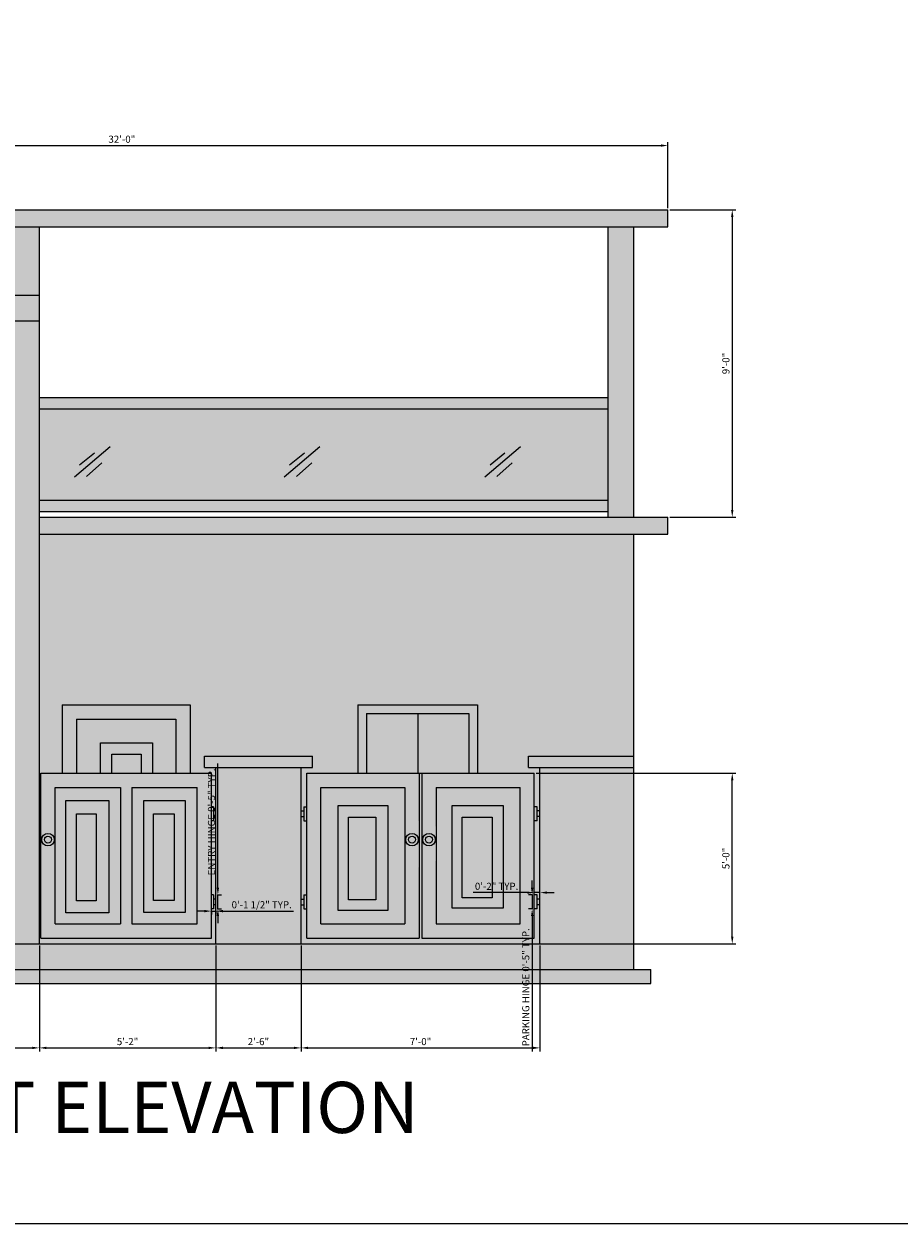
# Model space of a CAD drawing. Units: inches. Extents: x 2169 to 10664, y 1669 to 6352.
# Tile 2 of 17: x 2403 to 2710, y 1669 to 2091. Entities that reach past the tile are written whole.
import ezdxf

# ---------------------------------------------------------------- set-up
doc = ezdxf.new("R2010")
doc.units = ezdxf.units.IN
for name, color, linetype, lineweight in [('A-ANNO-DIMS', 3, 'Continuous', 18), ('A-ANNO-TITL', 3, 'Continuous', 25), ('A-ANNO-TTLB', 7, 'Continuous', 25), ('A-ELEV', 7, 'Continuous', 25), ('A-ELEV-CONC-PATT', 85, 'Continuous', 13), ('A-ELEV-GATE', 7, 'Continuous', 18), ('A-ELEV-GATE-PATT', 252, 'Continuous', 13), ('A-ELEV-OPEN', 7, 'Continuous', 18), ('A-ELEV-OPEN-PATT', 9, 'Continuous', 13), ('A-ELEV-PATT', 253, 'Continuous', 13)]:
    doc.layers.add(name, color=color, linetype=linetype, lineweight=lineweight)
doc.styles.get("Standard").update_dxf_attribs({"font": 'arial.ttf'})
doc.dimstyles.new('ISO-25', dxfattribs={"dimtxt": 2.5, "dimasz": 2.5, "dimexe": 1.25, "dimexo": 0.625, "dimtad": 1, "dimdec": 0, "dimlunit": 3, "dimtxsty": 'Standard', "dimcen": 2.5, "dimadec": 0, "dimazin": 0, "dimtfac": 1, "dimtdec": 0, "dimtmove": 0, "dimatfit": 3, "dimfxl": 1, "dimarcsym": 0})

# ---------------------------------------------------------------- blocks, each defined once
blk = doc.blocks.new('GLASS-MARK-A')
for p, q in [((0, 0), (12.55, 10.69)), ((1.85, 4.25), (7.07, 8.47)), ((4.25, 0.12), (9.7, 4.88))]:
    blk.add_line(p, q)
blk = doc.blocks.new('GATE-HINGE-1')
for p, q in [((0.75, 5), (0, 5)), ((0.75, 5), (0.75, 0)), ((0.75, 0), (0, 0)), ((1.5, 3.5), (0.75, 3.5)), ((1.5, 1.5), (0.75, 1.5))]:
    blk.add_line(p, q)
blk = doc.blocks.new('GATE-HINGE-2')
for p, q in [((1, 5), (2, 5)), ((1, 5), (1, 0)), ((0, 3.5), (1, 3.5)), ((0, 1.5), (1, 1.5)), ((1, 0), (2, 0))]:
    blk.add_line(p, q)
blk = doc.blocks.new('GATE-PULL-ROUND')
for radius in [2.2, 1.2]:
    blk.add_circle((2.21, 2.21), radius)
blk = doc.blocks.new('*D69')
at = {"layer": 'A-ANNO-DIMS', "color": 0, "lineweight": -2, "transparency": 16777216}
for p, q in [((2581.31, 1787.58), (2581.31, 1790.08)), ((2581.43, 1785.08), (2580.06, 1785.08)), ((2581.31, 1785.08), (2581.31, 1780.08)), ((2581.43, 1780.08), (2580.06, 1780.08)), ((2581.31, 1777.58), (2581.31, 1729.99))]:
    blk.add_line(p, q, dxfattribs=at)
at = {"layer": 'A-ANNO-DIMS', "color": 0, "transparency": 16777216}
for points in [[(2580.89, 1787.58), (2581.73, 1787.58), (2581.31, 1785.08)], [(2580.89, 1777.58), (2581.73, 1777.58), (2581.31, 1780.08)]]:
    blk.add_solid(points, dxfattribs=at)
at = {"layer": 'Defpoints', "color": 0, "transparency": 16777216}
for p in [(2582.06, 1785.08), (2581.31, 1780.08), (2582.06, 1780.08)]:
    blk.add_point(p, dxfattribs=at)
at = {"layer": 'A-ANNO-DIMS', "color": 0, "transparency": 16777216, "insert": (2579.39, 1752.54), "char_height": 2.5, "attachment_point": 5, "rotation": 90}
blk.add_mtext('PARKING HINGE 0\'-5" TYP.', dxfattribs=at)
blk = doc.blocks.new('*D70')
at = {"layer": 'A-ANNO-DIMS', "color": 0, "lineweight": -2, "transparency": 16777216}
for p, q in [((2579.56, 1785.83), (2560.57, 1785.83)), ((2582.06, 1785.7), (2582.06, 1787.08)), ((2584.06, 1785.83), (2582.06, 1785.83)), ((2584.06, 1785.7), (2584.06, 1787.08)), ((2586.56, 1785.83), (2589.06, 1785.83))]:
    blk.add_line(p, q, dxfattribs=at)
at = {"layer": 'A-ANNO-DIMS', "color": 0, "transparency": 16777216}
for points in [[(2579.56, 1786.24), (2579.56, 1785.41), (2582.06, 1785.83)], [(2586.56, 1786.24), (2586.56, 1785.41), (2584.06, 1785.83)]]:
    blk.add_solid(points, dxfattribs=at)
at = {"layer": 'Defpoints', "color": 0, "transparency": 16777216}
for p in [(2582.06, 1785.83), (2582.06, 1785.08), (2584.06, 1785.08)]:
    blk.add_point(p, dxfattribs=at)
at = {"layer": 'A-ANNO-DIMS', "color": 0, "transparency": 16777216, "insert": (2568.81, 1787.73), "char_height": 2.5, "attachment_point": 5}
blk.add_mtext('0\'-2" TYP.', dxfattribs=at)
blk = doc.blocks.new('*D79')
at = {"layer": 'A-ANNO-DIMS', "color": 0, "lineweight": -2, "transparency": 16777216}
for p, q in [((2470.81, 1787.58), (2470.81, 1831.27)), ((2470.68, 1785.08), (2472.06, 1785.08)), ((2470.81, 1780.08), (2470.81, 1785.08)), ((2470.68, 1780.08), (2472.06, 1780.08)), ((2470.81, 1777.58), (2470.81, 1775.08))]:
    blk.add_line(p, q, dxfattribs=at)
at = {"layer": 'A-ANNO-DIMS', "color": 0, "transparency": 16777216}
for points in [[(2470.39, 1787.58), (2471.23, 1787.58), (2470.81, 1785.08)], [(2470.39, 1777.58), (2471.23, 1777.58), (2470.81, 1780.08)]]:
    blk.add_solid(points, dxfattribs=at)
at = {"layer": 'Defpoints', "color": 0, "transparency": 16777216}
for p in [(2470.06, 1785.08), (2470.81, 1785.08), (2470.06, 1780.08)]:
    blk.add_point(p, dxfattribs=at)
at = {"layer": 'A-ANNO-DIMS', "color": 0, "transparency": 16777216, "insert": (2468.89, 1810.68), "char_height": 2.5, "attachment_point": 5, "rotation": 90}
blk.add_mtext('ENTRY HINGE 0\'-5" TYP.', dxfattribs=at)
blk = doc.blocks.new('*D80')
at = {"layer": 'A-ANNO-DIMS', "color": 0, "lineweight": -2, "transparency": 16777216}
for p, q in [((2466.06, 1779.33), (2463.56, 1779.33)), ((2468.56, 1779.45), (2468.56, 1778.08)), ((2468.56, 1779.33), (2470.06, 1779.33)), ((2470.06, 1779.45), (2470.06, 1778.08)), ((2472.56, 1779.33), (2497.37, 1779.33))]:
    blk.add_line(p, q, dxfattribs=at)
at = {"layer": 'A-ANNO-DIMS', "color": 0, "transparency": 16777216}
for points in [[(2466.06, 1779.74), (2466.06, 1778.91), (2468.56, 1779.33)], [(2472.56, 1779.74), (2472.56, 1778.91), (2470.06, 1779.33)]]:
    blk.add_solid(points, dxfattribs=at)
at = {"layer": 'Defpoints', "color": 0, "transparency": 16777216}
for p in [(2468.56, 1780.08), (2470.06, 1780.08), (2470.06, 1779.33)]:
    blk.add_point(p, dxfattribs=at)
at = {"layer": 'A-ANNO-DIMS', "color": 0, "transparency": 16777216, "insert": (2486.22, 1781.25), "char_height": 2.5, "attachment_point": 5}
blk.add_mtext('0\'-1 1/2" TYP.', dxfattribs=at)
blk = doc.blocks.new('*D93')
at = {"layer": 'A-ANNO-DIMS', "color": 0, "lineweight": -2, "transparency": 16777216}
for p, q in [((2245.06, 2026.47), (2245.06, 2049.69)), ((2247.56, 2048.44), (2626.56, 2048.44)), ((2629.06, 2026.47), (2629.06, 2049.69))]:
    blk.add_line(p, q, dxfattribs=at)
at = {"layer": 'A-ANNO-DIMS', "color": 0, "transparency": 16777216}
for points in [[(2247.56, 2048.86), (2247.56, 2048.03), (2245.06, 2048.44)], [(2626.56, 2048.86), (2626.56, 2048.03), (2629.06, 2048.44)]]:
    blk.add_solid(points, dxfattribs=at)
at = {"layer": 'Defpoints', "color": 0, "transparency": 16777216}
for p in [(2629.06, 2048.44), (2245.06, 2025.84), (2629.06, 2025.84)]:
    blk.add_point(p, dxfattribs=at)
at = {"layer": 'A-ANNO-DIMS', "color": 0, "transparency": 16777216, "insert": (2437.06, 2050.35), "char_height": 2.5, "attachment_point": 5}
blk.add_mtext('32\'-0"', dxfattribs=at)
blk = doc.blocks.new('*D94')
at = {"layer": 'A-ANNO-DIMS', "color": 0, "lineweight": -2, "transparency": 16777216}
for p, q in [((2629.68, 2025.84), (2652.91, 2025.84)), ((2651.66, 2023.34), (2651.66, 1920.34)), ((2629.68, 1917.84), (2652.91, 1917.84))]:
    blk.add_line(p, q, dxfattribs=at)
at = {"layer": 'A-ANNO-DIMS', "color": 0, "transparency": 16777216}
for points in [[(2651.24, 2023.34), (2652.08, 2023.34), (2651.66, 2025.84)], [(2651.24, 1920.34), (2652.08, 1920.34), (2651.66, 1917.84)]]:
    blk.add_solid(points, dxfattribs=at)
at = {"layer": 'Defpoints', "color": 0, "transparency": 16777216}
for p in [(2629.06, 2025.84), (2629.06, 1917.84), (2651.66, 1917.84)]:
    blk.add_point(p, dxfattribs=at)
at = {"layer": 'A-ANNO-DIMS', "color": 0, "transparency": 16777216, "insert": (2649.76, 1971.84), "char_height": 2.5, "attachment_point": 5, "rotation": 90}
blk.add_mtext('9\'-0"', dxfattribs=at)
blk = doc.blocks.new('*D97')
at = {"layer": 'A-ANNO-DIMS', "color": 0, "lineweight": -2, "transparency": 16777216}
for p, q in [((2375.55, 1820.07), (2375.55, 1729.99)), ((2408.06, 1767.22), (2408.06, 1729.99)), ((2378.05, 1731.24), (2405.56, 1731.24))]:
    blk.add_line(p, q, dxfattribs=at)
at = {"layer": 'A-ANNO-DIMS', "color": 0, "transparency": 16777216}
for points in [[(2378.05, 1731.66), (2378.05, 1730.83), (2375.55, 1731.24)], [(2405.56, 1731.66), (2405.56, 1730.83), (2408.06, 1731.24)]]:
    blk.add_solid(points, dxfattribs=at)
at = {"layer": 'Defpoints', "color": 0, "transparency": 16777216}
for p in [(2375.55, 1820.7), (2408.06, 1767.84), (2408.06, 1731.24)]:
    blk.add_point(p, dxfattribs=at)
at = {"layer": 'A-ANNO-DIMS', "color": 0, "transparency": 16777216, "insert": (2391.8, 1733.16), "char_height": 2.5, "attachment_point": 5}
blk.add_mtext('2\'-8 1/2"', dxfattribs=at)
blk = doc.blocks.new('*D98')
at = {"layer": 'A-ANNO-DIMS', "color": 0, "lineweight": -2, "transparency": 16777216}
for p, q in [((2408.06, 1767.22), (2408.06, 1729.99)), ((2470.06, 1767.22), (2470.06, 1729.99)), ((2410.56, 1731.24), (2467.56, 1731.24))]:
    blk.add_line(p, q, dxfattribs=at)
at = {"layer": 'A-ANNO-DIMS', "color": 0, "transparency": 16777216}
for points in [[(2410.56, 1731.66), (2410.56, 1730.83), (2408.06, 1731.24)], [(2467.56, 1731.66), (2467.56, 1730.83), (2470.06, 1731.24)]]:
    blk.add_solid(points, dxfattribs=at)
at = {"layer": 'Defpoints', "color": 0, "transparency": 16777216}
for p in [(2408.06, 1767.84), (2470.06, 1767.84), (2470.06, 1731.24)]:
    blk.add_point(p, dxfattribs=at)
at = {"layer": 'A-ANNO-DIMS', "color": 0, "transparency": 16777216, "insert": (2439.06, 1733.14), "char_height": 2.5, "attachment_point": 5}
blk.add_mtext('5\'-2"', dxfattribs=at)
blk = doc.blocks.new('*D99')
at = {"layer": 'A-ANNO-DIMS', "color": 0, "lineweight": -2, "transparency": 16777216}
for p, q in [((2470.06, 1767.22), (2470.06, 1729.99)), ((2500.06, 1767.22), (2500.06, 1729.99)), ((2472.56, 1731.24), (2497.56, 1731.24))]:
    blk.add_line(p, q, dxfattribs=at)
at = {"layer": 'A-ANNO-DIMS', "color": 0, "transparency": 16777216}
for points in [[(2472.56, 1731.66), (2472.56, 1730.83), (2470.06, 1731.24)], [(2497.56, 1731.66), (2497.56, 1730.83), (2500.06, 1731.24)]]:
    blk.add_solid(points, dxfattribs=at)
at = {"layer": 'Defpoints', "color": 0, "transparency": 16777216}
for p in [(2470.06, 1767.84), (2500.06, 1767.84), (2500.06, 1731.24)]:
    blk.add_point(p, dxfattribs=at)
at = {"layer": 'A-ANNO-DIMS', "color": 0, "transparency": 16777216, "insert": (2485.06, 1733.14), "char_height": 2.5, "attachment_point": 5}
blk.add_mtext('2\'-6"', dxfattribs=at)
blk = doc.blocks.new('*D100')
at = {"layer": 'A-ANNO-DIMS', "color": 0, "lineweight": -2, "transparency": 16777216}
for p, q in [((2500.06, 1767.22), (2500.06, 1729.99)), ((2584.06, 1767.22), (2584.06, 1729.99)), ((2502.56, 1731.24), (2581.56, 1731.24))]:
    blk.add_line(p, q, dxfattribs=at)
at = {"layer": 'A-ANNO-DIMS', "color": 0, "transparency": 16777216}
for points in [[(2502.56, 1731.66), (2502.56, 1730.83), (2500.06, 1731.24)], [(2581.56, 1731.66), (2581.56, 1730.83), (2584.06, 1731.24)]]:
    blk.add_solid(points, dxfattribs=at)
at = {"layer": 'Defpoints', "color": 0, "transparency": 16777216}
for p in [(2500.06, 1767.84), (2584.06, 1767.84), (2584.06, 1731.24)]:
    blk.add_point(p, dxfattribs=at)
at = {"layer": 'A-ANNO-DIMS', "color": 0, "transparency": 16777216, "insert": (2542.06, 1733.14), "char_height": 2.5, "attachment_point": 5}
blk.add_mtext('7\'-0"', dxfattribs=at)
blk = doc.blocks.new('*D101')
at = {"layer": 'A-ANNO-DIMS', "color": 0, "lineweight": -2, "transparency": 16777216}
for p, q in [((2582.68, 1827.84), (2652.91, 1827.84)), ((2651.66, 1770.34), (2651.66, 1825.34)), ((2584.68, 1767.84), (2652.91, 1767.84))]:
    blk.add_line(p, q, dxfattribs=at)
at = {"layer": 'A-ANNO-DIMS', "color": 0, "transparency": 16777216}
for points in [[(2651.24, 1825.34), (2652.08, 1825.34), (2651.66, 1827.84)], [(2651.24, 1770.34), (2652.08, 1770.34), (2651.66, 1767.84)]]:
    blk.add_solid(points, dxfattribs=at)
at = {"layer": 'Defpoints', "color": 0, "transparency": 16777216}
for p in [(2582.06, 1827.84), (2651.66, 1827.84), (2584.06, 1767.84)]:
    blk.add_point(p, dxfattribs=at)
at = {"layer": 'A-ANNO-DIMS', "color": 0, "transparency": 16777216, "insert": (2649.76, 1797.84), "char_height": 2.5, "attachment_point": 5, "rotation": 90}
blk.add_mtext('5\'-0"', dxfattribs=at)

msp = doc.modelspace()

# ---------------------------------------------------------------- hatches: boundary and pattern name
at = {"layer": 'A-ELEV-CONC-PATT'}
h = msp.add_hatch(dxfattribs=at)
h.set_pattern_fill('AR-CONC', color=256, scale=0.02)
h.paths.add_polyline_path([(2629.06, 2025.84), (2245.06, 2025.84), (2245.06, 2019.84), (2629.06, 2019.84)])
h.paths.add_polyline_path([(2257.06, 1917.84), (2245.06, 1917.84), (2245.06, 1911.84), (2257.06, 1911.84)])
h.paths.add_polyline_path([(2629.06, 1917.84), (2408.06, 1917.84), (2408.06, 1911.84), (2629.06, 1911.84)])
h = msp.add_hatch(dxfattribs=at)
h.set_pattern_fill('AR-CONC', color=256, scale=0.02)
h.paths.add_polyline_path([(2408.06, 1995.84), (2293.06, 1995.84), (2293.06, 1767.84), (2302.06, 1767.84), (2302.06, 1986.84), (2408.06, 1986.84)])
h = msp.add_hatch(dxfattribs=at)
h.set_pattern_fill('AR-CONC', color=256, scale=0.01)
h.paths.add_polyline_path([(2504.06, 1833.84), (2466.06, 1833.84), (2466.06, 1829.84), (2504.06, 1829.84)])
h.paths.add_polyline_path([(2617.06, 1833.84), (2580.06, 1833.84), (2580.06, 1829.84), (2617.06, 1829.84)])
at = {"layer": 'A-ELEV-GATE-PATT'}
h = msp.add_hatch(color=256, dxfattribs=at)
h.dxf.hatch_style = 1
h.paths.add_polyline_path([(2468.56, 1827.84), (2408.56, 1827.84), (2408.56, 1769.84), (2468.56, 1769.84)])
h.paths.add_polyline_path([(2413.56, 1822.84), (2436.56, 1822.84), (2436.56, 1774.84), (2413.56, 1774.84)], flags=16)
h.paths.add_polyline_path([(2417.37, 1818.23), (2432.48, 1818.23), (2432.48, 1778.74), (2417.37, 1778.74)], flags=0)
h.paths.add_polyline_path([(2421.12, 1813.58), (2428.06, 1813.58), (2428.06, 1782.94), (2421.12, 1782.94)], flags=0)
h.paths.add_polyline_path([(2413.27, 1804.47, -1), (2408.86, 1804.47, -1)], flags=16)
h.paths.add_polyline_path([(2412.27, 1804.47, -1), (2409.86, 1804.47, -1)], flags=0)
h.paths.add_polyline_path([(2440.56, 1822.84), (2463.56, 1822.84), (2463.56, 1774.84), (2440.56, 1774.84)], flags=16)
h.paths.add_polyline_path([(2444.81, 1818.23), (2459.3, 1818.23), (2459.3, 1778.87), (2444.81, 1778.87)], flags=0)
h.paths.add_polyline_path([(2448.24, 1813.58), (2455.4, 1813.58), (2455.4, 1783.07), (2448.24, 1783.07)], flags=0)
h.paths.add_polyline_path([(2541.56, 1827.84), (2502.06, 1827.84), (2502.06, 1769.84), (2541.56, 1769.84), (2541.27, 1804.47, -1), (2536.86, 1804.47), (2536.56, 1774.84), (2507.06, 1774.84), (2507.06, 1822.84), (2536.56, 1822.84), (2536.86, 1804.47, -1), (2541.27, 1804.47)])
h.paths.add_polyline_path([(2582.06, 1827.84), (2542.56, 1827.84), (2542.84, 1804.47, -1), (2547.25, 1804.47), (2547.56, 1822.84), (2577.06, 1822.84), (2577.06, 1774.84), (2547.56, 1774.84), (2547.25, 1804.47, -1), (2542.84, 1804.47), (2542.56, 1769.84), (2582.06, 1769.84)])
h.paths.add_polyline_path([(2530.6, 1816.44), (2513.06, 1816.44), (2513.06, 1779.59), (2530.6, 1779.59)], flags=17)
h.paths.add_polyline_path([(2516.79, 1812.39), (2526.37, 1812.39), (2526.37, 1783.31), (2516.79, 1783.31)], flags=16)
h.paths.add_polyline_path([(2571.11, 1816.44), (2553.14, 1816.44), (2553.14, 1780.32), (2571.11, 1780.32)], flags=17)
h.paths.add_polyline_path([(2556.75, 1812.38), (2567.23, 1812.38), (2567.23, 1784.01), (2556.75, 1784.01)], flags=16)
h.paths.add_polyline_path([(2459.3, 1818.23), (2444.81, 1818.23), (2444.81, 1778.87), (2459.3, 1778.87)], flags=0)
h.paths.add_polyline_path([(2432.48, 1818.23), (2417.37, 1818.23), (2417.37, 1778.74), (2432.48, 1778.74)], flags=0)
h = msp.add_hatch(color=256, dxfattribs=at)
h.dxf.hatch_style = 1
h.paths.add_polyline_path([(2436.56, 1822.84), (2413.56, 1822.84), (2413.56, 1774.84), (2436.56, 1774.84)])
h.paths.add_polyline_path([(2417.37, 1818.23), (2432.48, 1818.23), (2432.48, 1778.74), (2417.37, 1778.74)], flags=16)
h.paths.add_polyline_path([(2421.12, 1813.58), (2428.06, 1813.58), (2428.06, 1782.94), (2421.12, 1782.94)], flags=0)
h.paths.add_polyline_path([(2428.06, 1813.58), (2421.12, 1813.58), (2421.12, 1782.94), (2428.06, 1782.94)], flags=0)
h.paths.add_polyline_path([(2463.56, 1822.84), (2440.56, 1822.84), (2440.56, 1774.84), (2463.56, 1774.84)])
h.paths.add_polyline_path([(2459.3, 1818.23), (2459.3, 1778.87), (2444.81, 1778.87), (2444.81, 1818.23)], flags=16)
h.paths.add_polyline_path([(2448.24, 1813.58), (2455.4, 1813.58), (2455.4, 1783.07), (2448.24, 1783.07)], flags=0)
h.paths.add_polyline_path([(2536.56, 1822.84), (2507.06, 1822.84), (2507.06, 1774.84), (2536.56, 1774.84)])
h.paths.add_polyline_path([(2513.06, 1816.44), (2530.6, 1816.44), (2530.6, 1779.59), (2513.06, 1779.59)], flags=16)
h.paths.add_polyline_path([(2516.79, 1812.39), (2526.37, 1812.39), (2526.37, 1783.31), (2516.79, 1783.31)], flags=0)
h.paths.add_polyline_path([(2577.06, 1822.84), (2547.56, 1822.84), (2547.56, 1774.84), (2577.06, 1774.84)])
h.paths.add_polyline_path([(2553.14, 1816.44), (2571.11, 1816.44), (2571.11, 1780.32), (2553.14, 1780.32)], flags=16)
h.paths.add_polyline_path([(2556.75, 1812.38), (2567.23, 1812.38), (2567.23, 1784.01), (2556.75, 1784.01)], flags=0)
h = msp.add_hatch(color=256, dxfattribs=at)
h.dxf.hatch_style = 1
h.paths.add_polyline_path([(2432.48, 1818.23), (2417.37, 1818.23), (2417.37, 1778.74), (2432.48, 1778.74)])
h.paths.add_polyline_path([(2421.12, 1813.58), (2428.06, 1813.58), (2428.06, 1782.94), (2421.12, 1782.94)], flags=16)
h.paths.add_polyline_path([(2459.3, 1818.23), (2444.81, 1818.23), (2444.81, 1778.87), (2459.3, 1778.87)])
h.paths.add_polyline_path([(2448.24, 1813.58), (2455.4, 1813.58), (2455.4, 1783.07), (2448.24, 1783.07)], flags=16)
h.paths.add_polyline_path([(2469.31, 1816.03), (2468.56, 1816.03), (2468.56, 1811.03), (2469.31, 1811.03)])
h.paths.add_polyline_path([(2470.06, 1814.53), (2469.31, 1814.53), (2469.31, 1812.53), (2470.06, 1812.53)])
h.paths.add_polyline_path([(2469.31, 1785.08), (2468.56, 1785.08), (2468.56, 1780.08), (2469.31, 1780.08)])
h.paths.add_polyline_path([(2470.06, 1783.58), (2469.31, 1783.58), (2469.31, 1781.58), (2470.06, 1781.58)])
h.paths.add_polyline_path([(2502.06, 1816.03), (2501.06, 1816.03), (2501.06, 1811.03), (2502.06, 1811.03)])
h.paths.add_polyline_path([(2501.06, 1814.53), (2500.06, 1814.53), (2500.06, 1812.53), (2501.06, 1812.53)])
h.paths.add_polyline_path([(2502.06, 1785.08), (2501.06, 1785.08), (2501.06, 1780.08), (2502.06, 1780.08)])
h.paths.add_polyline_path([(2501.06, 1783.58), (2500.06, 1783.58), (2500.06, 1781.58), (2501.06, 1781.58)])
h.paths.add_polyline_path([(2584.06, 1783.58), (2583.06, 1783.58), (2583.06, 1781.58), (2584.06, 1781.58)])
h.paths.add_polyline_path([(2583.06, 1785.08), (2582.06, 1785.08), (2582.06, 1780.08), (2583.06, 1780.08)])
h.paths.add_polyline_path([(2583.06, 1816.03), (2582.06, 1816.03), (2582.06, 1811.03), (2583.06, 1811.03)])
h.paths.add_polyline_path([(2584.06, 1814.53), (2583.06, 1814.53), (2583.06, 1812.53), (2584.06, 1812.53)])
h = msp.add_hatch(color=256, dxfattribs=at)
h.dxf.hatch_style = 1
h.paths.add_polyline_path([(2428.06, 1813.58), (2421.12, 1813.58), (2421.12, 1782.94), (2428.06, 1782.94)])
h.paths.add_polyline_path([(2455.4, 1813.58), (2448.24, 1813.58), (2448.24, 1783.07), (2455.4, 1783.07)])
h.paths.add_polyline_path([(2526.37, 1812.39), (2516.79, 1812.39), (2516.79, 1783.31), (2526.37, 1783.31)])
h.paths.add_polyline_path([(2567.23, 1812.38), (2556.75, 1812.38), (2556.75, 1784.01), (2567.23, 1784.01)])
h = msp.add_hatch(color=256, dxfattribs=at)
h.dxf.hatch_style = 1
h.paths.add_polyline_path([(2408.86, 1804.47, 1), (2413.27, 1804.47, 1)])
h.paths.add_polyline_path([(2412.27, 1804.47, -1), (2409.86, 1804.47, -1)], flags=16)
h.paths.add_polyline_path([(2536.86, 1804.47, 1), (2541.27, 1804.47, 1)])
h.paths.add_polyline_path([(2540.27, 1804.47, -1), (2537.86, 1804.47, -1)], flags=16)
h.paths.add_polyline_path([(2542.84, 1804.47, 1), (2547.25, 1804.47, 1)])
h.paths.add_polyline_path([(2546.25, 1804.47, -1), (2543.84, 1804.47, -1)], flags=16)
h = msp.add_hatch(color=256, dxfattribs=at)
h.dxf.hatch_style = 1
h.paths.add_polyline_path([(2409.86, 1804.47, 1), (2412.27, 1804.47, 1)])
h.paths.add_polyline_path([(2540.27, 1804.47, 1), (2537.86, 1804.47, 1)])
h.paths.add_polyline_path([(2543.84, 1804.47, 1), (2546.25, 1804.47, 1)])
at = {"layer": 'A-ELEV-OPEN-PATT'}
h = msp.add_hatch(color=256, dxfattribs=at)
h.dxf.hatch_style = 1
h.paths.add_polyline_path([(2608.06, 1955.84), (2408.06, 1955.84), (2408.06, 1923.84), (2608.06, 1923.84)])
h.paths.add_polyline_path([(2371.55, 1970.13), (2321.5, 1970.13), (2321.5, 1870.03), (2329.06, 1870.03), (2329.06, 1876.03), (2338.06, 1876.03), (2338.06, 1882.03), (2347.06, 1882.03), (2347.06, 1888.03), (2356.06, 1888.03), (2356.06, 1894.03), (2365.06, 1894.03), (2365.06, 1900.03), (2371.55, 1900.03)])
h.paths.add_polyline_path([(2371.55, 1900.03), (2365.06, 1900.03), (2365.06, 1894.03), (2356.06, 1894.03), (2356.06, 1888.03), (2347.06, 1888.03), (2347.06, 1882.03), (2338.06, 1882.03), (2338.06, 1876.03), (2329.06, 1876.03), (2329.06, 1870.03), (2321.5, 1870.03), (2321.5, 1860.7), (2329.06, 1860.7), (2329.06, 1854.7), (2338.06, 1854.7), (2338.06, 1848.7), (2347.06, 1848.7), (2347.06, 1842.7), (2356.06, 1842.7), (2356.06, 1836.7), (2365.06, 1836.7), (2365.06, 1830.7), (2371.55, 1830.7)])
h.paths.add_polyline_path([(2365.06, 1836.7), (2356.06, 1836.7), (2356.06, 1842.7), (2347.06, 1842.7), (2347.06, 1848.7), (2338.06, 1848.7), (2338.06, 1854.7), (2329.06, 1854.7), (2329.06, 1860.7), (2321.5, 1860.7), (2321.5, 1824.7), (2371.55, 1824.7), (2371.55, 1830.7), (2365.06, 1830.7)])
h = msp.add_hatch(color=256, dxfattribs=at)
h.dxf.hatch_style = 1
h.paths.add_polyline_path([(2608.06, 1959.84), (2408.06, 1959.84), (2408.06, 1955.84), (2608.06, 1955.84)])
h.paths.add_polyline_path([(2608.06, 1923.84), (2408.06, 1923.84), (2408.06, 1919.84), (2608.06, 1919.84)])
h = msp.add_hatch(color=256, dxfattribs=at)
h.dxf.hatch_style = 1
h.paths.add_polyline_path([(2461.06, 1851.84), (2416.06, 1851.84), (2416.06, 1827.84), (2421.06, 1827.84), (2421.06, 1846.84), (2456.06, 1846.84), (2456.06, 1827.84), (2461.06, 1827.84)])
h.paths.add_polyline_path([(2447.86, 1838.51), (2429.59, 1838.51), (2429.59, 1827.84), (2433.59, 1827.84), (2433.59, 1834.51), (2443.86, 1834.51), (2443.86, 1827.84), (2447.86, 1827.84)], flags=17)
h = msp.add_hatch(color=256, dxfattribs=at)
h.dxf.hatch_style = 1
h.paths.add_polyline_path([(2562.06, 1851.84), (2520.06, 1851.84), (2520.06, 1827.84), (2523.06, 1827.84), (2523.06, 1848.84), (2559.06, 1848.84), (2559.06, 1827.84), (2562.06, 1827.84)])
h = msp.add_hatch(color=256, dxfattribs=at)
h.dxf.hatch_style = 1
h.paths.add_polyline_path([(2541.06, 1848.84), (2523.06, 1848.84), (2523.06, 1827.84), (2541.06, 1827.84)])
h.paths.add_polyline_path([(2559.06, 1848.84), (2541.06, 1848.84), (2541.06, 1827.84), (2541.56, 1827.84), (2542.56, 1827.84), (2559.06, 1827.84)])
h = msp.add_hatch(color=256, dxfattribs=at)
h.dxf.hatch_style = 1
h.paths.add_polyline_path([(2456.06, 1846.84), (2421.06, 1846.84), (2421.06, 1827.84), (2429.59, 1827.84), (2429.59, 1838.51), (2447.86, 1838.51), (2447.86, 1827.84), (2456.06, 1827.84)])
h.paths.add_polyline_path([(2443.86, 1834.51), (2433.59, 1834.51), (2433.59, 1827.84), (2443.86, 1827.84)], flags=17)
at = {"layer": 'A-ELEV-PATT'}
h = msp.add_hatch(color=256, dxfattribs=at)
h.dxf.hatch_style = 1
h.paths.add_polyline_path([(2408.06, 1986.84), (2302.06, 1986.84), (2302.06, 1767.84), (2408.06, 1767.84)], flags=17)
h.paths.add_polyline_path([(2375.55, 1820.7), (2317.5, 1820.7), (2317.5, 1974.13), (2375.55, 1974.13)], flags=16)
h.paths.add_polyline_path([(2371.55, 1824.7), (2321.5, 1824.7), (2321.5, 1970.13), (2371.55, 1970.13)], flags=0)
h.paths.add_polyline_path([(2293.06, 1995.84), (2408.06, 1995.84), (2408.06, 2019.84), (2257.06, 2019.84), (2257.06, 1767.84), (2293.06, 1767.84)])
h = msp.add_hatch(color=256, dxfattribs=at)
h.dxf.hatch_style = 1
h.paths.add_polyline_path([(2617.06, 2019.84), (2608.06, 2019.84), (2608.06, 1917.84), (2617.06, 1917.84)])
h = msp.add_hatch(color=256, dxfattribs=at)
h.dxf.hatch_style = 1
h.paths.add_polyline_path([(2617.06, 1911.84), (2408.06, 1911.84), (2408.06, 1767.84), (2470.06, 1767.84), (2470.06, 1781.58), (2469.31, 1781.58), (2469.31, 1780.08), (2468.56, 1780.08), (2468.56, 1769.84), (2408.56, 1769.84), (2408.56, 1827.84), (2416.06, 1827.84), (2416.06, 1851.84), (2461.06, 1851.84), (2461.06, 1827.84), (2468.56, 1827.84), (2468.56, 1816.03), (2469.31, 1816.03), (2469.31, 1814.53), (2470.06, 1814.53), (2470.06, 1829.84), (2466.06, 1829.84), (2466.06, 1833.84), (2504.06, 1833.84), (2504.06, 1829.84), (2500.06, 1829.84), (2500.06, 1814.53), (2501.06, 1814.53), (2501.06, 1816.03), (2502.06, 1816.03), (2502.06, 1827.84), (2520.06, 1827.84), (2520.06, 1851.84), (2562.06, 1851.84), (2562.06, 1827.84), (2582.06, 1827.84), (2582.06, 1816.03), (2583.06, 1816.03), (2583.06, 1814.53), (2584.06, 1814.53), (2584.06, 1829.84), (2580.06, 1829.84), (2580.06, 1833.84), (2617.06, 1833.84)])
h.paths.add_polyline_path([(2470.06, 1812.53), (2469.31, 1812.53), (2469.31, 1811.03), (2468.56, 1811.03), (2468.56, 1785.08), (2469.31, 1785.08), (2469.31, 1783.58), (2470.06, 1783.58)], flags=17)
h.paths.add_polyline_path([(2502.06, 1811.03), (2501.06, 1811.03), (2501.06, 1812.53), (2500.06, 1812.53), (2500.06, 1783.58), (2501.06, 1783.58), (2501.06, 1785.08), (2502.06, 1785.08)], flags=16)
h.paths.add_polyline_path([(2502.06, 1780.08), (2501.06, 1780.08), (2501.06, 1781.58), (2500.06, 1781.58), (2500.06, 1767.84), (2584.06, 1767.84), (2584.06, 1781.58), (2583.06, 1781.58), (2583.06, 1780.08), (2582.06, 1780.08), (2582.06, 1769.84), (2542.56, 1769.84), (2542.56, 1827.84), (2541.56, 1827.84), (2541.56, 1769.84), (2502.06, 1769.84)], flags=17)
h.paths.add_polyline_path([(2584.06, 1812.53), (2583.06, 1812.53), (2583.06, 1811.03), (2582.06, 1811.03), (2582.06, 1785.08), (2583.06, 1785.08), (2583.06, 1783.58), (2584.06, 1783.58)], flags=16)
h = msp.add_hatch(color=256, dxfattribs=at)
h.dxf.hatch_style = 1
h.paths.add_polyline_path([(2500.06, 1829.84), (2470.06, 1829.84), (2470.06, 1767.84), (2500.06, 1767.84)])
h.paths.add_polyline_path([(2617.06, 1829.84), (2584.06, 1829.84), (2584.06, 1767.84), (2617.06, 1767.84)])
h = msp.add_hatch(color=256, dxfattribs=at)
h.dxf.hatch_style = 1
h.paths.add_polyline_path([(2617.06, 1767.84), (2257.06, 1767.84), (2257.06, 1758.84), (2617.06, 1758.84)])
h = msp.add_hatch(color=256, dxfattribs=at)
h.dxf.hatch_style = 1
h.paths.add_polyline_path([(2623.06, 1758.84), (2251.06, 1758.84), (2251.06, 1753.84), (2623.06, 1753.84)])

# ---------------------------------------------------------------- linework, layer by layer
at = {"layer": 'A-ANNO-TTLB'}
msp.add_lwpolyline([(2169.45, 2838.28), (3251.13, 2838.28), (3251.13, 1669.34), (2169.45, 1669.34)], close=True, dxfattribs=at)
at = {"layer": 'A-ELEV'}
for p, q in [((2245.06, 2025.84), (2629.06, 2025.84)), ((2629.06, 2019.84), (2629.06, 2025.84)), ((2245.06, 2019.84), (2629.06, 2019.84)), ((2408.06, 1767.84), (2408.06, 2019.84)), ((2608.06, 1917.84), (2608.06, 2019.84)), ((2617.06, 1917.84), (2617.06, 2019.84)), ((2293.06, 1995.84), (2408.06, 1995.84)), ((2302.06, 1986.84), (2408.06, 1986.84)), ((2408.06, 1917.84), (2629.06, 1917.84)), ((2629.06, 1911.84), (2629.06, 1917.84)), ((2408.06, 1911.84), (2629.06, 1911.84)), ((2617.06, 1758.84), (2617.06, 1911.84)), ((2466.06, 1829.84), (2466.06, 1833.84)), ((2466.06, 1833.84), (2504.06, 1833.84)), ((2504.06, 1829.84), (2504.06, 1833.84)), ((2580.06, 1829.84), (2580.06, 1833.84)), ((2580.06, 1833.84), (2617.06, 1833.84)), ((2466.06, 1829.84), (2504.06, 1829.84)), ((2470.06, 1767.84), (2470.06, 1829.84)), ((2500.06, 1767.84), (2500.06, 1829.84)), ((2580.06, 1829.84), (2617.06, 1829.84)), ((2584.06, 1767.84), (2584.06, 1829.84)), ((2257.06, 1767.84), (2617.06, 1767.84)), ((2251.06, 1758.84), (2623.06, 1758.84)), ((2623.06, 1753.84), (2623.06, 1758.84)), ((2251.06, 1753.84), (2623.06, 1753.84))]:
    msp.add_line(p, q, dxfattribs=at)
at = {"layer": 'A-ELEV-GATE'}
for p, q in [((2408.56, 1827.84), (2468.56, 1827.84)), ((2408.56, 1769.84), (2408.56, 1827.84)), ((2468.56, 1769.84), (2468.56, 1827.84)), ((2502.06, 1769.84), (2502.06, 1827.84)), ((2502.06, 1827.84), (2541.56, 1827.84)), ((2541.56, 1827.84), (2541.56, 1769.84)), ((2541.56, 1827.84), (2542.56, 1827.84)), ((2542.56, 1827.84), (2542.56, 1769.84)), ((2542.56, 1827.84), (2582.06, 1827.84)), ((2582.06, 1769.84), (2582.06, 1827.84)), ((2413.56, 1822.84), (2436.56, 1822.84)), ((2413.56, 1774.84), (2413.56, 1822.84)), ((2436.56, 1822.84), (2436.56, 1774.84)), ((2440.56, 1822.84), (2440.56, 1774.84)), ((2440.56, 1822.84), (2463.56, 1822.84)), ((2463.56, 1774.84), (2463.56, 1822.84)), ((2507.06, 1774.84), (2507.06, 1822.84)), ((2507.06, 1822.84), (2536.56, 1822.84)), ((2536.56, 1822.84), (2536.56, 1774.84)), ((2547.56, 1822.84), (2547.56, 1774.84)), ((2547.56, 1822.84), (2577.06, 1822.84)), ((2577.06, 1774.84), (2577.06, 1822.84)), ((2413.56, 1774.84), (2436.56, 1774.84)), ((2440.56, 1774.84), (2463.56, 1774.84)), ((2507.06, 1774.84), (2536.56, 1774.84)), ((2547.56, 1774.84), (2577.06, 1774.84)), ((2408.56, 1769.84), (2468.56, 1769.84)), ((2502.06, 1769.84), (2541.56, 1769.84)), ((2542.56, 1769.84), (2582.06, 1769.84))]:
    msp.add_line(p, q, dxfattribs=at)
for points in [[(2417.37, 1818.23), (2432.48, 1818.23), (2432.48, 1778.74), (2417.37, 1778.74)], [(2444.81, 1818.23), (2459.3, 1818.23), (2459.3, 1778.87), (2444.81, 1778.87)], [(2513.06, 1816.44), (2530.6, 1816.44), (2530.6, 1779.59), (2513.06, 1779.59)], [(2553.14, 1816.44), (2571.11, 1816.44), (2571.11, 1780.32), (2553.14, 1780.32)], [(2421.12, 1813.58), (2428.06, 1813.58), (2428.06, 1782.94), (2421.12, 1782.94)], [(2448.24, 1813.58), (2455.4, 1813.58), (2455.4, 1783.07), (2448.24, 1783.07)], [(2516.79, 1812.39), (2526.37, 1812.39), (2526.37, 1783.31), (2516.79, 1783.31)], [(2556.75, 1812.38), (2567.23, 1812.38), (2567.23, 1784.01), (2556.75, 1784.01)]]:
    msp.add_lwpolyline(points, close=True, dxfattribs=at)
at = {"layer": 'A-ELEV-OPEN'}
for p, q in [((2408.06, 1959.84), (2608.06, 1959.84)), ((2408.06, 1955.84), (2608.06, 1955.84)), ((2408.06, 1923.84), (2608.06, 1923.84)), ((2408.06, 1919.84), (2608.06, 1919.84)), ((2416.06, 1851.84), (2461.06, 1851.84)), ((2416.06, 1851.84), (2416.06, 1827.84)), ((2461.06, 1851.84), (2461.06, 1827.84)), ((2520.06, 1851.84), (2562.06, 1851.84)), ((2520.06, 1851.84), (2520.06, 1827.84)), ((2523.06, 1848.84), (2523.06, 1827.84)), ((2523.06, 1848.84), (2559.06, 1848.84)), ((2541.06, 1848.84), (2541.06, 1827.84)), ((2559.06, 1848.84), (2559.06, 1827.84)), ((2562.06, 1851.84), (2562.06, 1827.84)), ((2421.06, 1846.84), (2456.06, 1846.84)), ((2421.06, 1846.84), (2421.06, 1827.84)), ((2456.06, 1846.84), (2456.06, 1827.84))]:
    msp.add_line(p, q, dxfattribs=at)
for points in [[(2429.59, 1827.84), (2429.59, 1838.51), (2447.86, 1838.51), (2447.86, 1827.84)], [(2433.59, 1827.84), (2433.59, 1834.51), (2443.86, 1834.51), (2443.86, 1827.84)]]:
    msp.add_lwpolyline(points, dxfattribs=at)

# ---------------------------------------------------------------- block references
at = {"layer": 'A-ELEV-GATE'}
for name, p in [('GATE-HINGE-1', (2468.56, 1811.03)), ('GATE-HINGE-2', (2500.06, 1811.04)), ('GATE-PULL-ROUND', (2408.86, 1802.26)), ('GATE-PULL-ROUND', (2536.86, 1802.26)), ('GATE-PULL-ROUND', (2542.84, 1802.26)), ('GATE-HINGE-1', (2468.56, 1780.08)), ('GATE-HINGE-2', (2500.06, 1780.08))]:
    msp.add_blockref(name, p, dxfattribs=at)
at = {"layer": 'A-ELEV-GATE', "rotation": 180}
for p in [(2584.06, 1816.03), (2584.06, 1785.08)]:
    msp.add_blockref('GATE-HINGE-2', p, dxfattribs=at)
at = {"layer": 'A-ELEV-OPEN'}
for p in [(2420.37, 1931.98), (2494.17, 1931.98), (2564.64, 1931.98)]:
    msp.add_blockref('GLASS-MARK-A', p, dxfattribs=at)

# ---------------------------------------------------------------- texts
at = {"layer": 'A-ANNO-TITL', "insert": (2326.86, 1719.32), "char_height": 18, "attachment_point": 1}
msp.add_mtext_dynamic_manual_height_columns('FRONT ELEVATION', width=700.4367, gutter_width=12.5, heights=[0], dxfattribs=at)

# ---------------------------------------------------------------- dimensions: what is measured, and where the dimension line sits
at = {"layer": 'A-ANNO-DIMS'}
for base, p1, p2, picture, middle in [((2629.06, 2048.44), (2245.06, 2025.84), (2629.06, 2025.84), '*D93', (2437.06, 2050.35)), ((2408.06, 1731.24), (2375.55, 1820.7), (2408.06, 1767.84), '*D97', (2391.8, 1733.16)), ((2470.06, 1731.24), (2408.06, 1767.84), (2470.06, 1767.84), '*D98', (2439.06, 1733.14)), ((2500.06, 1731.24), (2470.06, 1767.84), (2500.06, 1767.84), '*D99', (2485.06, 1733.14)), ((2584.06, 1731.24), (2500.06, 1767.84), (2584.06, 1767.84), '*D100', (2542.06, 1733.14))]:
    dim = msp.add_linear_dim(base=base, p1=p1, p2=p2, dimstyle='ISO-25', override={"dimdec": 1, "dimlfac": 1, "dimrnd": 0, "dimzin": 1, "dimdsep": 46, "dimlunit": 4, "dimfrac": 2}, dxfattribs=at)
    dim.commit()
    dim.dimension.update_dxf_attribs({"geometry": picture, "text_midpoint": middle})
for base, p1, p2, picture, middle in [((2651.66, 1917.84), (2629.06, 2025.84), (2629.06, 1917.84), '*D94', (2649.76, 1971.84)), ((2651.66, 1827.84), (2584.06, 1767.84), (2582.06, 1827.84), '*D101', (2649.76, 1797.84))]:
    dim = msp.add_linear_dim(base=base, p1=p1, p2=p2, angle=90, dimstyle='ISO-25', override={"dimdec": 1, "dimlfac": 1, "dimrnd": 0, "dimzin": 1, "dimdsep": 46, "dimlunit": 4, "dimfrac": 2}, dxfattribs=at)
    dim.commit()
    dim.dimension.update_dxf_attribs({"geometry": picture, "text_midpoint": middle})
for base, p1, p2, angle, text, picture, middle in [((2470.81, 1785.08), (2470.06, 1780.08), (2470.06, 1785.08), 90, 'ENTRY HINGE <> TYP.', '*D79', (2468.89, 1810.68)), ((2582.06, 1785.83), (2584.06, 1785.08), (2582.06, 1785.08), 180, '<> TYP.', '*D70', (2568.81, 1787.73)), ((2581.31, 1780.08), (2582.06, 1785.08), (2582.06, 1780.08), 270, 'PARKING HINGE <> TYP.', '*D69', (2579.39, 1752.54))]:
    dim = msp.add_linear_dim(base=base, p1=p1, p2=p2, angle=angle, text=text, dimstyle='ISO-25', override={"dimdec": 1, "dimlfac": 1, "dimrnd": 0, "dimzin": 1, "dimdsep": 46, "dimlunit": 4, "dimfrac": 2}, dxfattribs=at)
    dim.commit()
    dim.dimension.update_dxf_attribs({"geometry": picture, "text_midpoint": middle})
dim = msp.add_linear_dim(base=(2470.06, 1779.33), p1=(2468.56, 1780.08), p2=(2470.06, 1780.08), text='<> TYP.', dimstyle='ISO-25', override={"dimdec": 1, "dimlfac": 1, "dimrnd": 0, "dimzin": 1, "dimdsep": 46, "dimlunit": 4, "dimfrac": 2}, dxfattribs=at)
dim.commit()
dim.dimension.update_dxf_attribs({"geometry": '*D80', "text_midpoint": (2486.22, 1781.25)})

doc.saveas('drawing.dxf')
